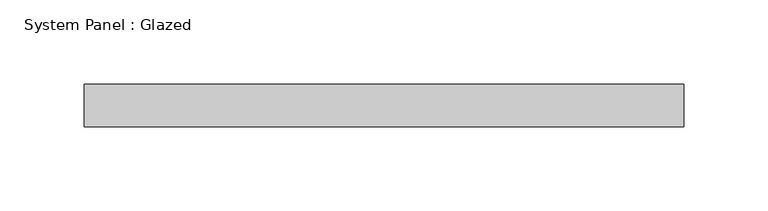
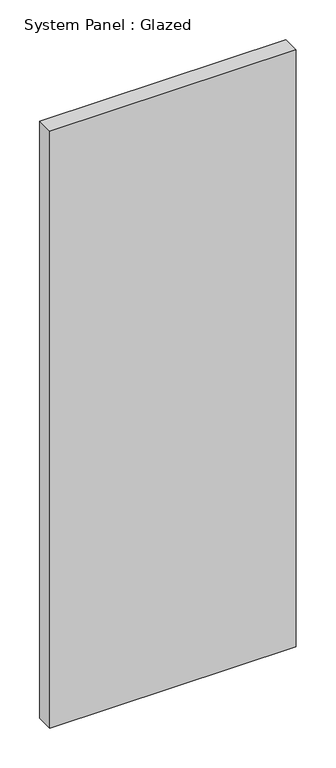
"""IFC4 building model written with IfcOpenShell, lengths in millimetres: plate geometry, System Panel : Glazed."""

from ifc_helpers import new_model, si_unit, origin, origin_with_axes, place, context, project, spatial, polyline, outline, extrude, source, transform, mapped, element, save


def system_panel_glazed_ac9e41bb(model_context):
    return source(origin(), model_context, "Body", "SweptSolid", [
        extrude(outline(polyline([(178.5541304, 19.05), (-178.5541304, 19.05), (-178.5541304, 44.45), (178.5541304, 44.45), (178.5541304, 19.05)])), origin_with_axes(), (0.0, 0.0, 1.0), 914.4),
    ])


if __name__ == "__main__":
    model = new_model("IFC4")
    model_context = context("Model", 3, world=origin())
    ifc_project = project(units=[si_unit("LENGTHUNIT", "METRE", prefix="MILLI")], contexts=[model_context])
    site = spatial("IfcSite", under=ifc_project)
    building = spatial("IfcBuilding", under=site)
    placement = place(None, origin())
    system_panel_glazed_shape = system_panel_glazed_ac9e41bb(model_context)
    element("IfcPlate", 1, ObjectType="System Panel : Glazed", at=placement, inside=building, context=model_context, shape_type="MappedRepresentation", body=[
        mapped(system_panel_glazed_shape, transform((0.0, 0.0, 0.0), x_axis=(1.0, 0.0, 0.0), y_axis=(0.0, 1.0, 0.0), z_axis=(0.0, 0.0, 1.0))),
    ])
    save(model, "model.ifc")

# Revit data of these elements
# Type "System Panel : Glazed"
#   Construction Type Id = "GSP4R"
#   Analytic Construction = "1/8 in Pilkington single glazing"
#   Visual Light Transmittance = 0.9
#   Solar Heat Gain Coefficient = 0.86
#   Heat Transfer Coefficient (U) = 1.18115 BTU/(h·ft²·°F)
# Element 1 (IfcPlate, "System Panel : Glazed")
#   Materials on its faces: "Glass"
# Materials
#   "Glass": class "Glass", colour RGB 0 128 192, transparency 0.75, Description = "Soda Lime Glass", Cost = 0
